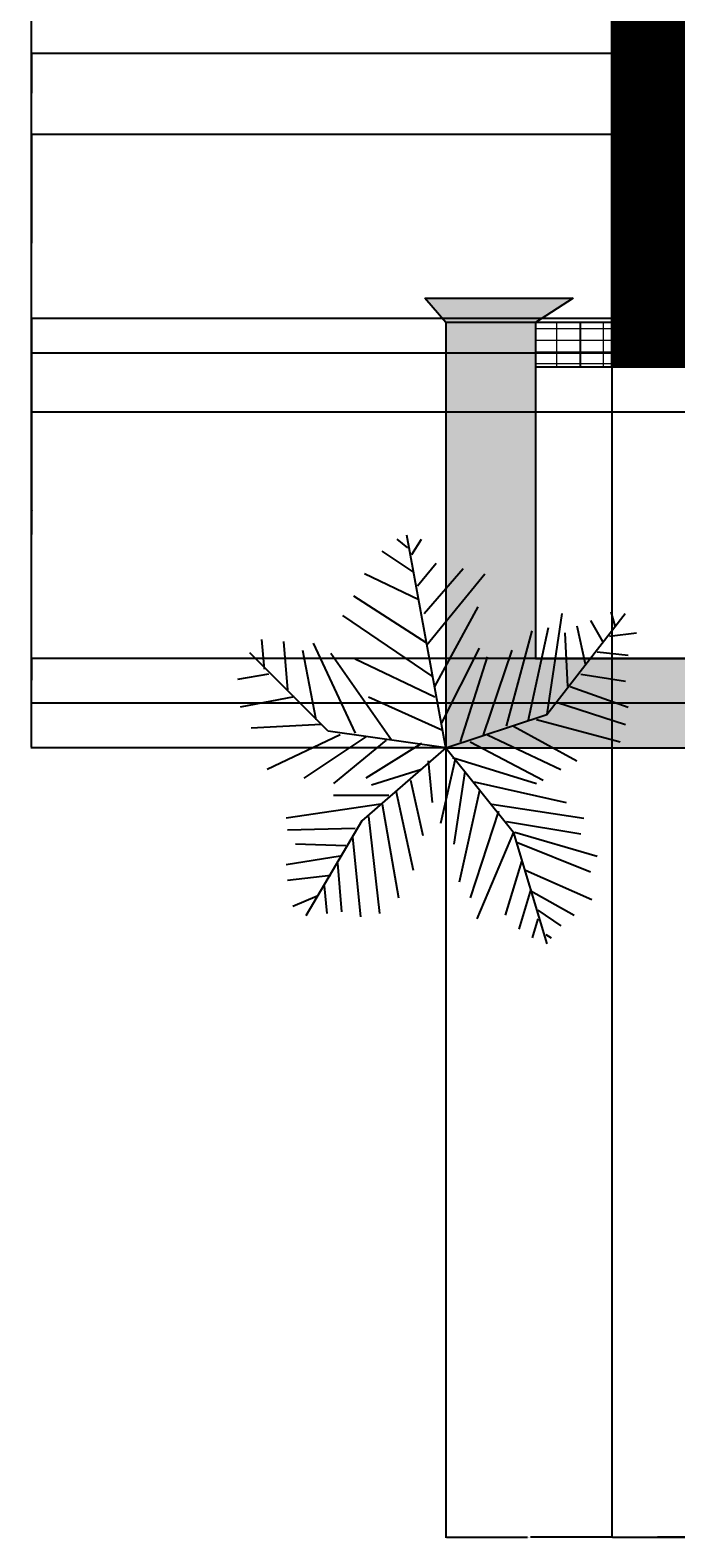
# Model space of a CAD drawing. Units: inches. Extents: x 484 to 1264, y 95 to 991.
# Tile 1 of 8: x 484 to 657, y 95 to 499. Entities that reach past the tile are written whole.
import ezdxf

# ---------------------------------------------------------------- set-up
doc = ezdxf.new("R2010")
doc.units = ezdxf.units.IN
doc.header["$MEASUREMENT"] = 0
for name, color, linetype, lineweight in [('A-ANNO-DIMS', 2, 'Continuous', 18), ('A-WALL', 7, 'Continuous', 35), ('L-FENC', 7, 'Continuous', 25), ('L-FENC-GRIL-PATT', 6, 'Continuous', 13)]:
    doc.layers.add(name, color=color, linetype=linetype, lineweight=lineweight)
for name, color, linetype, lineweight, true_color in [('A-ELEV-TRIM-PATT', 40, 'Continuous', 13, 0xe7c208), ('A-WALL-FRAM-PATT', 158, 'Continuous', 13, 0x131d3e), ('L-FENC-PATT', 34, 'Continuous', 13, 0xa25420)]:
    doc.layers.add(name, color=color, linetype=linetype, lineweight=lineweight, true_color=true_color)
doc.layers.add('TREES', color=92, linetype='Continuous')
doc.styles.get("Standard").update_dxf_attribs({"font": 'arial.ttf'})
doc.dimstyles.get("Standard").update_dxf_attribs({"dimtxt": 0.18, "dimasz": 0.18, "dimexe": 0.18, "dimexo": 0.0625, "dimgap": 0.09, "dimtad": 0, "dimtih": 1, "dimtoh": 1, "dimdec": 4, "dimzin": 0, "dimdsep": 46, "dimtxsty": 'Standard', "dimcen": 0.09, "dimadec": 0, "dimazin": 0, "dimtfac": 1, "dimtdec": 4, "dimtofl": 0, "dimtmove": 0, "dimatfit": 3, "dimfxl": 1, "dimtolj": 1, "dimtzin": 0, "dimarcsym": 0})

# ---------------------------------------------------------------- blocks, each defined once
blk = doc.blocks.new('*U2')
for p, q in [((0, 0), (-10.5, 57)), ((-8.737, 47.138), (-17.069, 52.711)), ((-10.186, 53.64), (-13.084, 55.962)), ((-9.099, 51.782), (-6.563, 55.962)), ((-7.65, 43.423), (-2.578, 49.46)), ((-7.288, 39.707), (-21.778, 46.673)), ((-5.839, 35.992), (4.667, 48.067)), ((-5.114, 27.632), (10.463, 46.673)), ((-5.114, 28.097), (-24.676, 40.636)), ((-2.941, 16.486), (8.652, 37.85)), ((44.153, 36.456), (45.239, 32.741)), ((-3.665, 19.273), (-27.574, 35.527)), ((27, 9), (48, 36)), ((27.127, 9.056), (31.112, 35.992)), ((35.096, 32.741), (37.27, 22.524)), ((38.719, 34.134), (41.979, 28.561)), ((-48.585, 21.131), (-49.309, 29.026)), ((-43.513, 28.561), (-42.427, 15.558)), ((16.259, 5.805), (23.142, 31.348)), ((22.055, 7.198), (27.489, 32.277)), ((31.836, 30.883), (32.561, 16.486)), ((43.791, 29.954), (51.036, 30.883)), ((-31.5, 4.5), (-52.5, 25.5)), ((-38.442, 26.239), (-34.819, 7.663)), ((-35.544, 28.097), (-24.314, 3.947)), ((-14.533, 2.09), (-30.834, 25.31)), ((-1.129, 6.734), (9.014, 26.704)), ((3.942, 1.625), (11.187, 24.381)), ((10.101, 3.483), (17.708, 26.239)), ((40.53, 25.775), (48.862, 24.846)), ((-24.314, 23.917), (-2.941, 13.7)), ((-47.498, 19.737), (-55.83, 18.344)), ((33.285, 16.486), (48.862, 10.913)), ((36.183, 19.737), (48.137, 17.88)), ((-40.615, 13.7), (-55.105, 10.913)), ((-20.691, 13.7), (-1.129, 4.876)), ((29.662, 12.307), (48.137, 6.269)), ((0, 0), (27, 9)), ((-33.37, 6.269), (-52.207, 5.34)), ((0, 0), (-31.5, 4.5)), ((18.07, 5.805), (35.096, -3.483)), ((24.229, 7.663), (46.688, 1.625)), ((-28.299, 3.483), (-47.86, -5.805)), ((-21.416, 3.018), (-38.079, -8.128)), ((-15.982, 2.09), (-30.11, -9.521)), ((0, 0), (-22.5, -19.5)), ((-6.563, 1.161), (-21.416, -8.128)), ((0, 0), (18, -22.5)), ((6.478, 1.625), (26.04, -8.592)), ((11.187, 3.483), (30.749, -5.805)), ((-4.752, -3.483), (-3.665, -14.629)), ((2.493, -3.019), (-1.491, -20.202)), ((1.769, -2.555), (24.229, -9.521)), ((-6.563, -5.805), (-19.967, -9.985)), ((5.029, -6.27), (2.131, -25.775)), ((-13.446, -11.378), (-8.737, -32.741)), ((-9.461, -8.592), (-6.201, -23.453)), ((9.014, -11.378), (3.58, -35.992)), ((7.565, -9.056), (32.198, -14.629)), ((-17.431, -15.094), (-42.789, -18.809)), ((-15.257, -12.772), (-30.11, -12.772)), ((-17.069, -15.094), (-12.721, -40.172)), ((12.274, -15.094), (36.907, -18.809)), ((-22.5, -19.5), (-37.5, -45)), ((-20.691, -18.345), (-17.793, -44.352)), ((14.085, -16.951), (6.478, -40.172)), ((16.259, -19.738), (36.183, -22.989)), ((-24.314, -21.596), (-42.427, -22.06)), ((-25.038, -23.918), (-22.865, -45.281)), ((18.07, -22.524), (8.289, -45.745)), ((18, -22.5), (27, -52.5)), ((18.433, -22.524), (40.53, -29.026)), ((-26.849, -26.24), (-40.253, -25.775)), ((19.157, -25.311), (38.719, -33.206)), ((-28.299, -29.026), (-42.789, -31.348)), ((-29.023, -30.884), (-27.936, -43.887)), ((20.244, -30.419), (15.897, -44.816)), ((-30.834, -34.135), (-42.427, -35.528)), ((21.331, -32.741), (39.081, -40.636)), ((-34.457, -39.708), (-40.978, -42.494)), ((-32.646, -36.921), (-31.921, -44.352)), ((22.78, -37.85), (19.519, -48.532)), ((22.78, -38.314), (34.372, -44.816)), ((24.591, -43.423), (30.749, -47.603)), ((24.591, -45.745), (23.142, -50.854)), ((26.764, -49.925), (28.213, -50.854))]:
    blk.add_line(p, q)
blk = doc.blocks.new('FENCE-PIER-CAP')
for p, q in [((5.63, 0), (0, 6.48)), ((0, 6.48), (39.71, 6.48)), ((39.71, 6.48), (29.63, 0))]:
    blk.add_line(p, q)
blk = doc.blocks.new('*D16')
at = {"layer": 'A-ANNO-DIMS', "color": 0, "lineweight": -2, "transparency": 16777216}
for p, q in [((639.81, 408.32), (639.81, 94.79)), ((999.81, 318.32), (999.81, 94.79)), ((639.99, 94.97), (819.53, 94.97)), ((999.63, 94.97), (820.1, 94.97))]:
    blk.add_line(p, q, dxfattribs=at)
at = {"layer": 'A-ANNO-DIMS', "color": 0, "transparency": 16777216}
for points in [[(639.99, 95), (639.99, 94.94), (639.81, 94.97)], [(999.63, 95), (999.63, 94.94), (999.81, 94.97)]]:
    blk.add_solid(points, dxfattribs=at)
at = {"layer": 'Defpoints', "color": 0, "transparency": 16777216}
for p in [(639.81, 408.38), (999.81, 318.38), (999.81, 94.97)]:
    blk.add_point(p, dxfattribs=at)
at = {"layer": 'A-ANNO-DIMS', "color": 0, "transparency": 16777216, "insert": (819.81, 94.97), "char_height": 0.18, "attachment_point": 5}
blk.add_mtext('\\A1;360', dxfattribs=at)
blk = doc.blocks.new('*D17')
at = {"layer": 'A-ANNO-DIMS', "color": 0, "lineweight": -2, "transparency": 16777216}
for p, q in [((709.01, 950.08), (484.15, 950.08)), ((484.33, 949.9), (484.33, 628.41)), ((484.33, 306.56), (484.33, 628.05)), ((595.26, 306.38), (484.15, 306.38))]:
    blk.add_line(p, q, dxfattribs=at)
at = {"layer": 'A-ANNO-DIMS', "color": 0, "transparency": 16777216}
for points in [[(484.3, 949.9), (484.36, 949.9), (484.33, 950.08)], [(484.3, 306.56), (484.36, 306.56), (484.33, 306.38)]]:
    blk.add_solid(points, dxfattribs=at)
at = {"layer": 'Defpoints', "color": 0, "transparency": 16777216}
for p in [(484.33, 950.08), (709.07, 950.08), (595.32, 306.38)]:
    blk.add_point(p, dxfattribs=at)
at = {"layer": 'A-ANNO-DIMS', "color": 0, "transparency": 16777216, "insert": (484.33, 628.23), "char_height": 0.18, "attachment_point": 5}
blk.add_mtext('\\A1;643.7', dxfattribs=at)
blk = doc.blocks.new('*D18')
at = {"layer": 'A-ANNO-DIMS', "color": 0, "lineweight": -2, "transparency": 16777216}
for p, q in [((999.88, 501.38), (1264.08, 501.38)), ((1263.9, 501.2), (1263.9, 404.07)), ((1263.9, 306.56), (1263.9, 403.7)), ((595.38, 306.38), (1264.08, 306.38))]:
    blk.add_line(p, q, dxfattribs=at)
at = {"layer": 'A-ANNO-DIMS', "color": 0, "transparency": 16777216}
for points in [[(1263.87, 501.2), (1263.93, 501.2), (1263.9, 501.38)], [(1263.87, 306.56), (1263.93, 306.56), (1263.9, 306.38)]]:
    blk.add_solid(points, dxfattribs=at)
at = {"layer": 'Defpoints', "color": 0, "transparency": 16777216}
for p in [(999.81, 501.38), (1263.9, 501.38), (595.32, 306.38)]:
    blk.add_point(p, dxfattribs=at)
at = {"layer": 'A-ANNO-DIMS', "color": 0, "transparency": 16777216, "insert": (1263.9, 403.88), "char_height": 0.18, "attachment_point": 5}
blk.add_mtext('\\A1;195', dxfattribs=at)
blk = doc.blocks.new('*D21')
at = {"layer": 'A-ANNO-DIMS', "color": 0, "lineweight": -2, "transparency": 16777216}
for p, q in [((639.81, 408.32), (639.81, 94.79)), ((595.32, 306.32), (595.32, 94.79)), ((595.5, 94.97), (617.17, 94.97)), ((639.63, 94.97), (617.97, 94.97))]:
    blk.add_line(p, q, dxfattribs=at)
at = {"layer": 'A-ANNO-DIMS', "color": 0, "transparency": 16777216}
for points in [[(595.5, 95), (595.5, 94.94), (595.32, 94.97)], [(639.63, 95), (639.63, 94.94), (639.81, 94.97)]]:
    blk.add_solid(points, dxfattribs=at)
at = {"layer": 'Defpoints', "color": 0, "transparency": 16777216}
for p in [(639.81, 408.38), (595.32, 306.38), (639.81, 94.97)]:
    blk.add_point(p, dxfattribs=at)
at = {"layer": 'A-ANNO-DIMS', "color": 0, "transparency": 16777216, "insert": (617.57, 94.97), "char_height": 0.18, "attachment_point": 5}
blk.add_mtext('\\A1;44.49', dxfattribs=at)
blk = doc.blocks.new('*D33')
at = {"layer": 'A-ANNO-DIMS', "color": 0, "lineweight": -2, "transparency": 16777216}
for p, q in [((639.81, 930.32), (639.81, 94.79)), ((663.81, 810.32), (663.81, 94.79)), ((639.99, 94.97), (651.59, 94.97)), ((663.63, 94.97), (652.03, 94.97))]:
    blk.add_line(p, q, dxfattribs=at)
at = {"layer": 'A-ANNO-DIMS', "color": 0, "transparency": 16777216}
for points in [[(639.99, 95), (639.99, 94.94), (639.81, 94.97)], [(663.63, 95), (663.63, 94.94), (663.81, 94.97)]]:
    blk.add_solid(points, dxfattribs=at)
at = {"layer": 'Defpoints', "color": 0, "transparency": 16777216}
for p in [(639.81, 930.38), (663.81, 810.38), (663.81, 94.97)]:
    blk.add_point(p, dxfattribs=at)
at = {"layer": 'A-ANNO-DIMS', "color": 0, "transparency": 16777216, "insert": (651.81, 94.97), "char_height": 0.18, "attachment_point": 5}
blk.add_mtext('\\A1;24', dxfattribs=at)
blk = doc.blocks.new('*D47')
at = {"layer": 'A-ANNO-DIMS', "color": 0, "lineweight": -2, "transparency": 16777216}
for p, q in [((779.84, 470.76), (484.15, 470.76)), ((484.33, 470.58), (484.33, 441.64)), ((484.33, 412.34), (484.33, 441.28)), ((779.84, 412.16), (484.15, 412.16))]:
    blk.add_line(p, q, dxfattribs=at)
at = {"layer": 'A-ANNO-DIMS', "color": 0, "transparency": 16777216}
for points in [[(484.3, 470.58), (484.36, 470.58), (484.33, 470.76)], [(484.3, 412.34), (484.36, 412.34), (484.33, 412.16)]]:
    blk.add_solid(points, dxfattribs=at)
at = {"layer": 'Defpoints', "color": 0, "transparency": 16777216}
for p in [(484.33, 470.76), (779.91, 470.76), (779.91, 412.16)]:
    blk.add_point(p, dxfattribs=at)
at = {"layer": 'A-ANNO-DIMS', "color": 0, "transparency": 16777216, "insert": (484.33, 441.46), "char_height": 0.18, "attachment_point": 5}
blk.add_mtext('\\A1;58.6', dxfattribs=at)
blk = doc.blocks.new('*D48')
at = {"layer": 'A-ANNO-DIMS', "color": 0, "lineweight": -2, "transparency": 16777216}
for p, q in [((831.75, 492.38), (484.15, 492.38)), ((484.33, 492.2), (484.33, 481.76)), ((484.33, 470.94), (484.33, 481.39)), ((779.84, 470.76), (484.15, 470.76))]:
    blk.add_line(p, q, dxfattribs=at)
at = {"layer": 'A-ANNO-DIMS', "color": 0, "transparency": 16777216}
for points in [[(484.3, 492.2), (484.36, 492.2), (484.33, 492.38)], [(484.3, 470.94), (484.36, 470.94), (484.33, 470.76)]]:
    blk.add_solid(points, dxfattribs=at)
at = {"layer": 'Defpoints', "color": 0, "transparency": 16777216}
for p in [(484.33, 492.38), (831.81, 492.38), (779.91, 470.76)]:
    blk.add_point(p, dxfattribs=at)
at = {"layer": 'A-ANNO-DIMS', "color": 0, "transparency": 16777216, "insert": (484.33, 481.57), "char_height": 0.18, "attachment_point": 5}
blk.add_mtext('\\A1;21.62', dxfattribs=at)
blk = doc.blocks.new('*D51')
at = {"layer": 'A-ANNO-DIMS', "color": 0, "lineweight": -2, "transparency": 16777216}
for p, q in [((869.55, 421.47), (484.15, 421.47)), ((484.33, 421.29), (484.33, 370.11)), ((484.33, 318.56), (484.33, 369.75)), ((855.75, 318.38), (484.15, 318.38))]:
    blk.add_line(p, q, dxfattribs=at)
at = {"layer": 'A-ANNO-DIMS', "color": 0, "transparency": 16777216}
for points in [[(484.3, 421.29), (484.36, 421.29), (484.33, 421.47)], [(484.3, 318.56), (484.36, 318.56), (484.33, 318.38)]]:
    blk.add_solid(points, dxfattribs=at)
at = {"layer": 'Defpoints', "color": 0, "transparency": 16777216}
for p in [(484.33, 421.47), (869.61, 421.47), (855.81, 318.38)]:
    blk.add_point(p, dxfattribs=at)
at = {"layer": 'A-ANNO-DIMS', "color": 0, "transparency": 16777216, "insert": (484.33, 369.93), "char_height": 0.18, "attachment_point": 5}
blk.add_mtext('\\A1;103.09', dxfattribs=at)
blk = doc.blocks.new('*D58')
at = {"layer": 'A-ANNO-DIMS', "color": 0, "lineweight": -2, "transparency": 16777216}
for p, q in [((855.75, 396.38), (484.15, 396.38)), ((484.33, 396.2), (484.33, 363.57)), ((484.33, 330.56), (484.33, 363.2)), ((855.75, 330.38), (484.15, 330.38))]:
    blk.add_line(p, q, dxfattribs=at)
at = {"layer": 'A-ANNO-DIMS', "color": 0, "transparency": 16777216}
for points in [[(484.3, 396.2), (484.36, 396.2), (484.33, 396.38)], [(484.3, 330.56), (484.36, 330.56), (484.33, 330.38)]]:
    blk.add_solid(points, dxfattribs=at)
at = {"layer": 'Defpoints', "color": 0, "transparency": 16777216}
for p in [(484.33, 396.38), (855.81, 396.38), (855.81, 330.38)]:
    blk.add_point(p, dxfattribs=at)
at = {"layer": 'A-ANNO-DIMS', "color": 0, "transparency": 16777216, "insert": (484.33, 363.38), "char_height": 0.18, "attachment_point": 5}
blk.add_mtext('\\A1;66', dxfattribs=at)
blk = doc.blocks.new('*D60')
at = {"layer": 'A-ANNO-DIMS', "color": 0, "lineweight": -2, "transparency": 16777216}
for p, q in [((855.75, 330.38), (484.15, 330.38)), ((484.33, 330.2), (484.33, 324.56)), ((484.33, 318.56), (484.33, 324.2)), ((855.75, 318.38), (484.15, 318.38))]:
    blk.add_line(p, q, dxfattribs=at)
at = {"layer": 'A-ANNO-DIMS', "color": 0, "transparency": 16777216}
for points in [[(484.3, 330.2), (484.36, 330.2), (484.33, 330.38)], [(484.3, 318.56), (484.36, 318.56), (484.33, 318.38)]]:
    blk.add_solid(points, dxfattribs=at)
at = {"layer": 'Defpoints', "color": 0, "transparency": 16777216}
for p in [(484.33, 330.38), (855.81, 330.38), (855.81, 318.38)]:
    blk.add_point(p, dxfattribs=at)
at = {"layer": 'A-ANNO-DIMS', "color": 0, "transparency": 16777216, "insert": (484.33, 324.38), "char_height": 0.18, "attachment_point": 5}
blk.add_mtext('\\A1;12', dxfattribs=at)

msp = doc.modelspace()

# ---------------------------------------------------------------- hatches: boundary and pattern name
at = {"layer": 'A-ELEV-TRIM-PATT'}
h = msp.add_hatch(color=256, dxfattribs=at)
h.dxf.hatch_style = 1
h.paths.add_polyline_path([(629.3986, 426.86), (589.6936, 426.86), (595.3221, 420.3846), (619.3221, 420.3846)])
edge = h.paths.add_edge_path()
edge.add_line((857.8147, 421.9731), (857.8147, 421.9373))
edge.add_ellipse((838.7195, 429.7418), major_axis=(-35.8241, 0), ratio=0.25748145, start_angle=157.76958, end_angle=158.416192)
edge.add_line((858.2614, 422.011), (865.8912, 426.9141))
edge.add_line((865.8912, 426.9141), (826.1862, 426.9141))
edge.add_line((826.1862, 426.9141), (831.8617, 420.3846))
edge.add_line((831.8617, 420.3846), (855.7305, 420.3846))
edge.add_line((855.7305, 420.3846), (856.3445, 420.7792))
edge.add_line((856.3445, 420.7792), (857.8147, 421.9731))
h.paths.add_polyline_path([(1009.8912, 426.86), (970.1862, 426.86), (975.8147, 420.3846), (999.8147, 420.3846)])
h.paths.add_polyline_path([(857.8147, 421.7239), (856.3445, 420.7792), (855.8147, 420.3489), (855.8147, 396.3846), (857.8147, 396.3846)])
edge = h.paths.add_edge_path()
edge.add_ellipse((838.7195, 448.4615), major_axis=(-35.8241, 0), ratio=0.25748145, start_angle=154.631086, end_angle=157.76958, ccw=False)
edge.add_line((855.8147, 440.3555), (855.8147, 437.8478))
edge.add_ellipse((838.7195, 429.7418), major_axis=(-35.8241, 0), ratio=0.25748145, start_angle=202.23042, end_angle=205.368914, ccw=False)
edge.add_line((857.8147, 437.5462), (857.8147, 440.6571))
edge = h.paths.add_edge_path()
edge.add_line((907.4984, 442.7783), (866.9359, 442.7783))
edge.add_ellipse((838.7195, 448.4615), major_axis=(-35.8241, 0), ratio=0.25748145, start_angle=158.813461, end_angle=168.611984, ccw=False)
edge.add_line((858.542, 440.7783), (905.4984, 440.7783))
edge.add_line((905.4984, 440.7783), (905.4984, 418.7562))
edge.add_line((905.4984, 418.7562), (907.4984, 416.8218))
edge.add_line((907.4984, 416.8218), (907.4984, 442.7783))
at = {"layer": 'A-WALL-FRAM-PATT'}
h = msp.add_hatch(dxfattribs=at)
h.set_pattern_fill('ANSI31', color=256)
h.paths.add_polyline_path([(999.8147, 810.3846), (831.8147, 810.3846), (831.8147, 501.3846), (999.8147, 501.3846), (999.8147, 537.3846), (855.8147, 537.3846), (855.8147, 705.3846), (999.8147, 705.3846)])
h.paths.add_polyline_path([(850.1752, 699.3334), (850.1752, 681.6082), (840.6401, 681.6082), (840.6401, 699.3334)], flags=16)
h.paths.add_polyline_path([(850.9809, 648.8447), (850.9809, 628.2143), (839.9453, 628.2143), (839.9453, 648.8447)], flags=16)
h.paths.add_polyline_path([(849.208, 595.8059), (849.208, 577.6654), (838.5284, 577.6654), (838.5284, 595.8059)], flags=16)
h.paths.add_polyline_path([(663.8147, 906.3846), (709.0683, 906.3846), (709.0683, 930.3846), (639.8147, 930.3846), (639.8147, 408.3846), (663.8147, 408.3846)])
h.paths.add_polyline_path([(885.8147, 930.3846), (775.2587, 930.3846), (775.2587, 906.3846), (885.8147, 906.3846)])
h.paths.add_polyline_path([(760.8695, 930.3846), (750.5092, 930.3846), (750.5092, 906.3846), (760.8695, 906.3846)])
h.paths.add_polyline_path([(736.12, 930.3846), (723.4575, 930.3846), (723.4575, 906.3846), (736.12, 906.3846)])
at = {"layer": 'L-FENC-GRIL-PATT'}
h = msp.add_hatch(dxfattribs=at)
h.set_pattern_fill('GRATE', color=256, scale=100)
h.paths.add_polyline_path([(974.8147, 396.3846), (927.8147, 396.3846), (927.8147, 330.3846), (974.8147, 330.3846)])
h.paths.add_polyline_path([(903.8147, 396.3846), (855.8147, 396.3846), (855.8147, 330.3846), (903.8147, 330.3846)])
h.paths.add_polyline_path([(819.8147, 420.3846), (807.8147, 420.3846), (807.8147, 408.3846), (819.8147, 408.3846)])
h.paths.add_polyline_path([(807.8147, 420.3846), (795.8147, 420.3846), (795.8147, 408.3846), (807.8147, 408.3846)])
h.paths.add_polyline_path([(795.8147, 420.3846), (783.8147, 420.3846), (783.8147, 408.3846), (795.8147, 408.3846)])
h.paths.add_polyline_path([(831.8147, 420.3846), (819.8147, 420.3846), (819.8147, 408.3846), (831.8147, 408.3846)])
h.paths.add_polyline_path([(783.8147, 420.3846), (779.9105, 420.3846), (779.9105, 412.138), (771.8147, 412.138), (771.8147, 408.3846), (783.8147, 408.3846)])
h.paths.add_polyline_path([(777.9105, 420.3846), (771.8147, 420.3846), (771.8147, 414.138), (777.9105, 414.138)], flags=17)
h.paths.add_polyline_path([(723.8147, 420.3846), (711.8147, 420.3846), (711.8147, 408.3846), (723.8147, 408.3846)])
h.paths.add_polyline_path([(711.8147, 420.3846), (699.8147, 420.3846), (699.8147, 408.3846), (711.8147, 408.3846)])
h.paths.add_polyline_path([(699.8147, 420.3846), (687.8147, 420.3846), (687.8147, 408.3846), (699.8147, 408.3846)])
h.paths.add_polyline_path([(687.8147, 420.3846), (675.8147, 420.3846), (675.8147, 408.3846), (687.8147, 408.3846)])
h.paths.add_polyline_path([(675.8147, 420.3846), (663.8147, 420.3846), (663.8147, 408.3846), (675.8147, 408.3846)])
h.paths.add_polyline_path([(639.8147, 420.3846), (631.3221, 420.3846), (631.3221, 408.3846), (639.8147, 408.3846)])
h.paths.add_polyline_path([(631.3221, 420.3846), (619.3221, 420.3846), (619.3221, 408.3846), (631.3221, 408.3846)])
at = {"layer": 'L-FENC-PATT'}
h = msp.add_hatch(color=256, dxfattribs=at)
h.dxf.hatch_style = 1
h.paths.add_polyline_path([(619.3221, 420.3846), (595.3221, 420.3846), (595.3221, 306.3846), (855.8147, 306.3846), (855.8147, 420.3846), (831.8147, 420.3846), (831.8147, 330.3846), (771.8147, 330.3846), (771.8147, 420.3846), (723.8147, 420.3846), (723.8147, 330.3846), (619.3221, 330.3846)])
h.paths.add_polyline_path([(999.8147, 420.3846), (975.8147, 420.3846), (975.8147, 318.3846), (999.8147, 318.3846)])

# ---------------------------------------------------------------- linework, layer by layer
at = {"layer": 'A-WALL'}
msp.add_line((639.8147, 930.3846), (639.8147, 408.3846), dxfattribs=at)
at = {"layer": 'L-FENC'}
for p, q in [((595.3221, 420.3846), (595.3221, 306.3846)), ((639.8147, 420.3846), (595.3221, 420.3846)), ((619.3221, 420.3846), (619.3221, 330.3846)), ((631.3221, 420.3846), (631.3221, 408.3846)), ((723.8147, 408.3846), (619.3221, 408.3846)), ((619.3221, 330.3846), (723.8147, 330.3846)), ((595.3221, 306.3846), (855.8147, 306.3846))]:
    msp.add_line(p, q, dxfattribs=at)

# ---------------------------------------------------------------- block references
msp.add_blockref('FENCE-PIER-CAP', (589.6936, 420.3846), dxfattribs=at)
at = {"layer": 'TREES'}
msp.add_blockref('*U2', (595.3221, 306.3846), dxfattribs=at)

# ---------------------------------------------------------------- dimensions: what is measured, and where the dimension line sits
at = {"layer": 'A-ANNO-DIMS'}
for base, p1, p2, override, picture, middle in [((484.3261, 950.079), (595.3221, 306.3846), (709.0683, 950.079), {"dimdec": 1, "dimlfac": 1, "dimrnd": 0, "dimzin": 0, "dimdsep": 46, "dimlunit": 2}, '*D17', (484.3261, 628.2318)), ((1263.9032, 501.3846), (595.3221, 306.3846), (999.8147, 501.3846), {"dimdec": 0, "dimlfac": 1, "dimrnd": 0, "dimzin": 0, "dimdsep": 46, "dimlunit": 2}, '*D18', (1263.9032, 403.8846)), ((484.3261, 492.3846), (779.9074, 470.7627), (831.8147, 492.3846), {"dimdec": 2, "dimlfac": 1, "dimrnd": 0, "dimzin": 0, "dimdsep": 46, "dimlunit": 2}, '*D48', (484.3261, 481.5737)), ((484.3261, 470.7627), (779.9074, 412.1588), (779.9074, 470.7627), {"dimdec": 1, "dimlfac": 1, "dimrnd": 0, "dimzin": 0, "dimdsep": 46, "dimlunit": 2}, '*D47', (484.3261, 441.4608)), ((484.3261, 421.4725), (855.8147, 318.3846), (869.6148, 421.4725), {"dimdec": 2, "dimlfac": 1, "dimrnd": 0, "dimzin": 0, "dimdsep": 46, "dimlunit": 2}, '*D51', (484.3261, 369.9286)), ((484.3261, 396.3846), (855.8147, 330.3846), (855.8147, 396.3846), {"dimdec": 0, "dimlfac": 1, "dimrnd": 0, "dimzin": 0, "dimdsep": 46, "dimlunit": 2}, '*D58', (484.3261, 363.3846)), ((484.3261, 330.3846), (855.8147, 318.3846), (855.8147, 330.3846), {"dimdec": 0, "dimlfac": 1, "dimrnd": 0, "dimzin": 0, "dimdsep": 46, "dimlunit": 2}, '*D60', (484.3261, 324.3846))]:
    dim = msp.add_linear_dim(base=base, p1=p1, p2=p2, angle=90, dimstyle='Standard', override=override, dxfattribs=at)
    dim.commit()
    dim.dimension.update_dxf_attribs({"geometry": picture, "text_midpoint": middle})
for base, p1, p2, override, picture, middle in [((663.8147, 94.9714), (639.8147, 930.3846), (663.8147, 810.3846), {"dimdec": 0, "dimlfac": 1, "dimrnd": 0, "dimzin": 0, "dimdsep": 46, "dimlunit": 2}, '*D33', (651.8147, 94.9714)), ((639.8147, 94.9714), (595.3221, 306.3846), (639.8147, 408.3846), {"dimdec": 2, "dimlfac": 1, "dimrnd": 0, "dimzin": 0, "dimdsep": 46, "dimlunit": 2}, '*D21', (617.5684, 94.9714)), ((999.8147, 94.9714), (639.8147, 408.3846), (999.8147, 318.3846), {"dimdec": 0, "dimlfac": 1, "dimrnd": 0, "dimzin": 0, "dimdsep": 46, "dimlunit": 2}, '*D16', (819.8147, 94.9714))]:
    dim = msp.add_linear_dim(base=base, p1=p1, p2=p2, dimstyle='Standard', override=override, dxfattribs=at)
    dim.commit()
    dim.dimension.update_dxf_attribs({"geometry": picture, "text_midpoint": middle})

doc.saveas('drawing.dxf')
